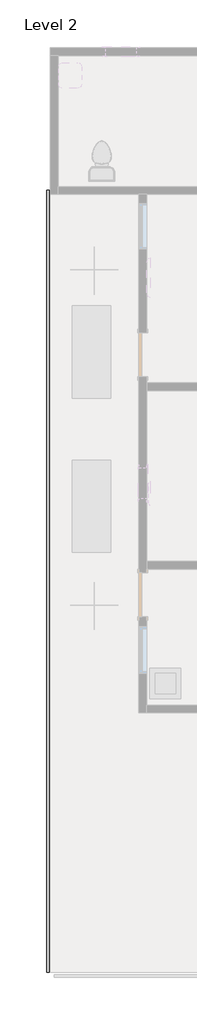
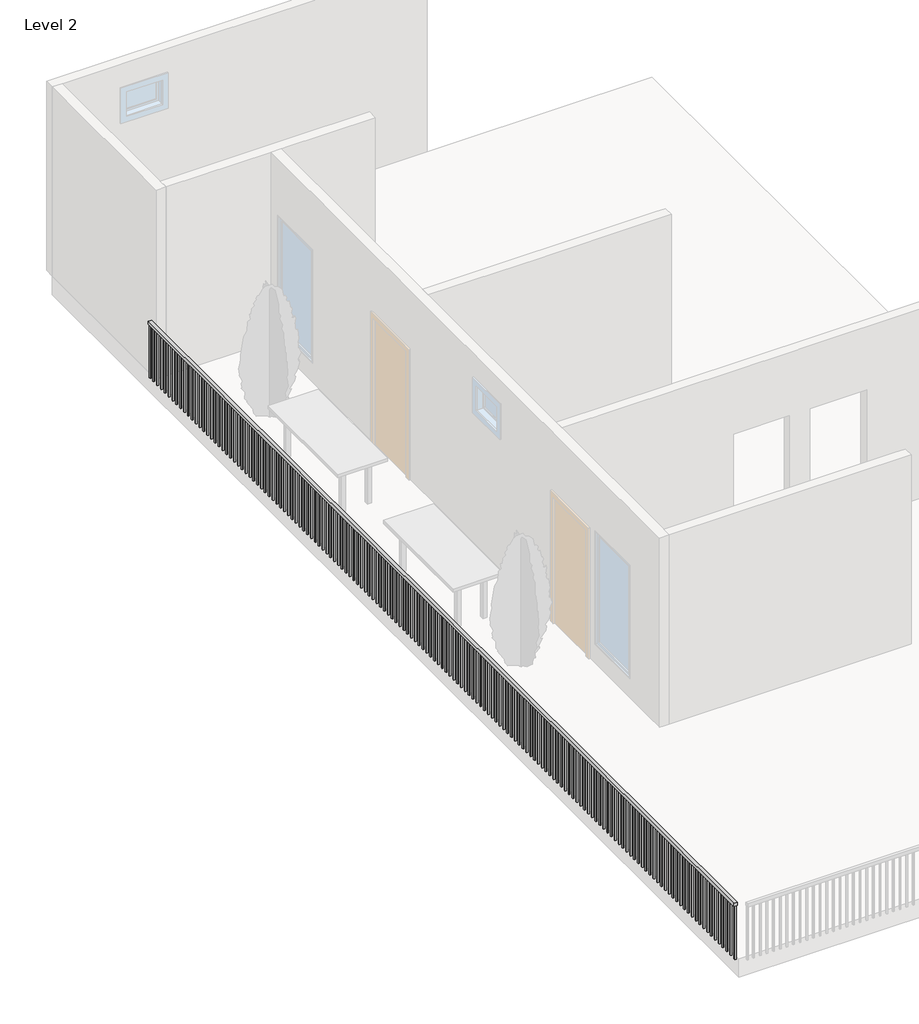
# One storey, part 3 of 4: 1 railing.
"""IFC4 building model written with IfcOpenShell, lengths in millimetres."""

from ifc_helpers import new_model, si_unit, frame, origin, place, context, project, spatial, polyline, outline, extrude, element, save

model = new_model("IFC4")

# Units and contexts
model_context = context("Model", 3, world=origin())
ifc_project = project(units=[si_unit("LENGTHUNIT", "METRE", prefix="MILLI")], contexts=[model_context])

# Site, building, storey
site = spatial("IfcSite", under=ifc_project)
building = spatial("IfcBuilding", under=site)
storey = spatial("IfcBuildingStorey", under=building, Name="Level 2", Elevation=3048.0)

# Railing
placement = place(None, origin())
element("IfcRailing", 1, ObjectType="Handrail - Rectangular", at=placement, inside=storey, context=model_context, shape_type="SweptSolid", body=[
    extrude(outline(polyline([(-12111.260887, 10860.7910469), (-12060.460887, 10860.7910469), (-12060.460887, -4607.8089531), (-12111.260887, -4607.8089531), (-12111.260887, 10860.7910469)])), frame((0.0, 0.0, 3911.6), z_axis=(0.0, 0.0, 1.0), x_axis=(1.0, 0.0, 0.0)), (0.0, 0.0, 1.0), 50.8),
    extrude(outline(polyline([(-12095.385887, -4572.8839531), (-12076.335887, -4572.8839531), (-12076.335887, -4591.9339531), (-12095.385887, -4591.9339531), (-12095.385887, -4572.8839531)])), frame((0.0, 0.0, 3048.0), z_axis=(0.0, 0.0, 1.0), x_axis=(1.0, 0.0, 0.0)), (0.0, 0.0, 1.0), 863.6),
    extrude(outline(polyline([(-12095.385887, -4471.2839531), (-12076.335887, -4471.2839531), (-12076.335887, -4490.3339531), (-12095.385887, -4490.3339531), (-12095.385887, -4471.2839531)])), frame((0.0, 0.0, 3048.0), z_axis=(0.0, 0.0, 1.0), x_axis=(1.0, 0.0, 0.0)), (0.0, 0.0, 1.0), 863.6),
    extrude(outline(polyline([(-12095.385887, -4369.6839531), (-12076.335887, -4369.6839531), (-12076.335887, -4388.7339531), (-12095.385887, -4388.7339531), (-12095.385887, -4369.6839531)])), frame((0.0, 0.0, 3048.0), z_axis=(0.0, 0.0, 1.0), x_axis=(1.0, 0.0, 0.0)), (0.0, 0.0, 1.0), 863.6),
    extrude(outline(polyline([(-12095.385887, -4268.0839531), (-12076.335887, -4268.0839531), (-12076.335887, -4287.1339531), (-12095.385887, -4287.1339531), (-12095.385887, -4268.0839531)])), frame((0.0, 0.0, 3048.0), z_axis=(0.0, 0.0, 1.0), x_axis=(1.0, 0.0, 0.0)), (0.0, 0.0, 1.0), 863.6),
    extrude(outline(polyline([(-12095.385887, -4166.4839531), (-12076.335887, -4166.4839531), (-12076.335887, -4185.5339531), (-12095.385887, -4185.5339531), (-12095.385887, -4166.4839531)])), frame((0.0, 0.0, 3048.0), z_axis=(0.0, 0.0, 1.0), x_axis=(1.0, 0.0, 0.0)), (0.0, 0.0, 1.0), 863.6),
    extrude(outline(polyline([(-12095.385887, -4064.8839531), (-12076.335887, -4064.8839531), (-12076.335887, -4083.9339531), (-12095.385887, -4083.9339531), (-12095.385887, -4064.8839531)])), frame((0.0, 0.0, 3048.0), z_axis=(0.0, 0.0, 1.0), x_axis=(1.0, 0.0, 0.0)), (0.0, 0.0, 1.0), 863.6),
    extrude(outline(polyline([(-12095.385887, -3963.2839531), (-12076.335887, -3963.2839531), (-12076.335887, -3982.3339531), (-12095.385887, -3982.3339531), (-12095.385887, -3963.2839531)])), frame((0.0, 0.0, 3048.0), z_axis=(0.0, 0.0, 1.0), x_axis=(1.0, 0.0, 0.0)), (0.0, 0.0, 1.0), 863.6),
    extrude(outline(polyline([(-12095.385887, -3861.6839531), (-12076.335887, -3861.6839531), (-12076.335887, -3880.7339531), (-12095.385887, -3880.7339531), (-12095.385887, -3861.6839531)])), frame((0.0, 0.0, 3048.0), z_axis=(0.0, 0.0, 1.0), x_axis=(1.0, 0.0, 0.0)), (0.0, 0.0, 1.0), 863.6),
    extrude(outline(polyline([(-12095.385887, -3760.0839531), (-12076.335887, -3760.0839531), (-12076.335887, -3779.1339531), (-12095.385887, -3779.1339531), (-12095.385887, -3760.0839531)])), frame((0.0, 0.0, 3048.0), z_axis=(0.0, 0.0, 1.0), x_axis=(1.0, 0.0, 0.0)), (0.0, 0.0, 1.0), 863.6),
    extrude(outline(polyline([(-12095.385887, -3658.4839531), (-12076.335887, -3658.4839531), (-12076.335887, -3677.5339531), (-12095.385887, -3677.5339531), (-12095.385887, -3658.4839531)])), frame((0.0, 0.0, 3048.0), z_axis=(0.0, 0.0, 1.0), x_axis=(1.0, 0.0, 0.0)), (0.0, 0.0, 1.0), 863.6),
    extrude(outline(polyline([(-12095.385887, -3556.8839531), (-12076.335887, -3556.8839531), (-12076.335887, -3575.9339531), (-12095.385887, -3575.9339531), (-12095.385887, -3556.8839531)])), frame((0.0, 0.0, 3048.0), z_axis=(0.0, 0.0, 1.0), x_axis=(1.0, 0.0, 0.0)), (0.0, 0.0, 1.0), 863.6),
    extrude(outline(polyline([(-12095.385887, -3455.2839531), (-12076.335887, -3455.2839531), (-12076.335887, -3474.3339531), (-12095.385887, -3474.3339531), (-12095.385887, -3455.2839531)])), frame((0.0, 0.0, 3048.0), z_axis=(0.0, 0.0, 1.0), x_axis=(1.0, 0.0, 0.0)), (0.0, 0.0, 1.0), 863.6),
    extrude(outline(polyline([(-12095.385887, -3353.6839531), (-12076.335887, -3353.6839531), (-12076.335887, -3372.7339531), (-12095.385887, -3372.7339531), (-12095.385887, -3353.6839531)])), frame((0.0, 0.0, 3048.0), z_axis=(0.0, 0.0, 1.0), x_axis=(1.0, 0.0, 0.0)), (0.0, 0.0, 1.0), 863.6),
    extrude(outline(polyline([(-12095.385887, -3252.0839531), (-12076.335887, -3252.0839531), (-12076.335887, -3271.1339531), (-12095.385887, -3271.1339531), (-12095.385887, -3252.0839531)])), frame((0.0, 0.0, 3048.0), z_axis=(0.0, 0.0, 1.0), x_axis=(1.0, 0.0, 0.0)), (0.0, 0.0, 1.0), 863.6),
    extrude(outline(polyline([(-12095.385887, -3150.4839531), (-12076.335887, -3150.4839531), (-12076.335887, -3169.5339531), (-12095.385887, -3169.5339531), (-12095.385887, -3150.4839531)])), frame((0.0, 0.0, 3048.0), z_axis=(0.0, 0.0, 1.0), x_axis=(1.0, 0.0, 0.0)), (0.0, 0.0, 1.0), 863.6),
    extrude(outline(polyline([(-12095.385887, -3048.8839531), (-12076.335887, -3048.8839531), (-12076.335887, -3067.9339531), (-12095.385887, -3067.9339531), (-12095.385887, -3048.8839531)])), frame((0.0, 0.0, 3048.0), z_axis=(0.0, 0.0, 1.0), x_axis=(1.0, 0.0, 0.0)), (0.0, 0.0, 1.0), 863.6),
    extrude(outline(polyline([(-12095.385887, -2947.2839531), (-12076.335887, -2947.2839531), (-12076.335887, -2966.3339531), (-12095.385887, -2966.3339531), (-12095.385887, -2947.2839531)])), frame((0.0, 0.0, 3048.0), z_axis=(0.0, 0.0, 1.0), x_axis=(1.0, 0.0, 0.0)), (0.0, 0.0, 1.0), 863.6),
    extrude(outline(polyline([(-12095.385887, -2845.6839531), (-12076.335887, -2845.6839531), (-12076.335887, -2864.7339531), (-12095.385887, -2864.7339531), (-12095.385887, -2845.6839531)])), frame((0.0, 0.0, 3048.0), z_axis=(0.0, 0.0, 1.0), x_axis=(1.0, 0.0, 0.0)), (0.0, 0.0, 1.0), 863.6),
    extrude(outline(polyline([(-12095.385887, -2744.0839531), (-12076.335887, -2744.0839531), (-12076.335887, -2763.1339531), (-12095.385887, -2763.1339531), (-12095.385887, -2744.0839531)])), frame((0.0, 0.0, 3048.0), z_axis=(0.0, 0.0, 1.0), x_axis=(1.0, 0.0, 0.0)), (0.0, 0.0, 1.0), 863.6),
    extrude(outline(polyline([(-12095.385887, -2642.4839531), (-12076.335887, -2642.4839531), (-12076.335887, -2661.5339531), (-12095.385887, -2661.5339531), (-12095.385887, -2642.4839531)])), frame((0.0, 0.0, 3048.0), z_axis=(0.0, 0.0, 1.0), x_axis=(1.0, 0.0, 0.0)), (0.0, 0.0, 1.0), 863.6),
    extrude(outline(polyline([(-12095.385887, -2540.8839531), (-12076.335887, -2540.8839531), (-12076.335887, -2559.9339531), (-12095.385887, -2559.9339531), (-12095.385887, -2540.8839531)])), frame((0.0, 0.0, 3048.0), z_axis=(0.0, 0.0, 1.0), x_axis=(1.0, 0.0, 0.0)), (0.0, 0.0, 1.0), 863.6),
    extrude(outline(polyline([(-12095.385887, -2439.2839531), (-12076.335887, -2439.2839531), (-12076.335887, -2458.3339531), (-12095.385887, -2458.3339531), (-12095.385887, -2439.2839531)])), frame((0.0, 0.0, 3048.0), z_axis=(0.0, 0.0, 1.0), x_axis=(1.0, 0.0, 0.0)), (0.0, 0.0, 1.0), 863.6),
    extrude(outline(polyline([(-12095.385887, -2337.6839531), (-12076.335887, -2337.6839531), (-12076.335887, -2356.7339531), (-12095.385887, -2356.7339531), (-12095.385887, -2337.6839531)])), frame((0.0, 0.0, 3048.0), z_axis=(0.0, 0.0, 1.0), x_axis=(1.0, 0.0, 0.0)), (0.0, 0.0, 1.0), 863.6),
    extrude(outline(polyline([(-12095.385887, -2236.0839531), (-12076.335887, -2236.0839531), (-12076.335887, -2255.1339531), (-12095.385887, -2255.1339531), (-12095.385887, -2236.0839531)])), frame((0.0, 0.0, 3048.0), z_axis=(0.0, 0.0, 1.0), x_axis=(1.0, 0.0, 0.0)), (0.0, 0.0, 1.0), 863.6),
    extrude(outline(polyline([(-12095.385887, -2134.4839531), (-12076.335887, -2134.4839531), (-12076.335887, -2153.5339531), (-12095.385887, -2153.5339531), (-12095.385887, -2134.4839531)])), frame((0.0, 0.0, 3048.0), z_axis=(0.0, 0.0, 1.0), x_axis=(1.0, 0.0, 0.0)), (0.0, 0.0, 1.0), 863.6),
    extrude(outline(polyline([(-12095.385887, -2032.8839531), (-12076.335887, -2032.8839531), (-12076.335887, -2051.9339531), (-12095.385887, -2051.9339531), (-12095.385887, -2032.8839531)])), frame((0.0, 0.0, 3048.0), z_axis=(0.0, 0.0, 1.0), x_axis=(1.0, 0.0, 0.0)), (0.0, 0.0, 1.0), 863.6),
    extrude(outline(polyline([(-12095.385887, -1931.2839531), (-12076.335887, -1931.2839531), (-12076.335887, -1950.3339531), (-12095.385887, -1950.3339531), (-12095.385887, -1931.2839531)])), frame((0.0, 0.0, 3048.0), z_axis=(0.0, 0.0, 1.0), x_axis=(1.0, 0.0, 0.0)), (0.0, 0.0, 1.0), 863.6),
    extrude(outline(polyline([(-12095.385887, -1829.6839531), (-12076.335887, -1829.6839531), (-12076.335887, -1848.7339531), (-12095.385887, -1848.7339531), (-12095.385887, -1829.6839531)])), frame((0.0, 0.0, 3048.0), z_axis=(0.0, 0.0, 1.0), x_axis=(1.0, 0.0, 0.0)), (0.0, 0.0, 1.0), 863.6),
    extrude(outline(polyline([(-12095.385887, -1728.0839531), (-12076.335887, -1728.0839531), (-12076.335887, -1747.1339531), (-12095.385887, -1747.1339531), (-12095.385887, -1728.0839531)])), frame((0.0, 0.0, 3048.0), z_axis=(0.0, 0.0, 1.0), x_axis=(1.0, 0.0, 0.0)), (0.0, 0.0, 1.0), 863.6),
    extrude(outline(polyline([(-12095.385887, -1626.4839531), (-12076.335887, -1626.4839531), (-12076.335887, -1645.5339531), (-12095.385887, -1645.5339531), (-12095.385887, -1626.4839531)])), frame((0.0, 0.0, 3048.0), z_axis=(0.0, 0.0, 1.0), x_axis=(1.0, 0.0, 0.0)), (0.0, 0.0, 1.0), 863.6),
    extrude(outline(polyline([(-12095.385887, -1524.8839531), (-12076.335887, -1524.8839531), (-12076.335887, -1543.9339531), (-12095.385887, -1543.9339531), (-12095.385887, -1524.8839531)])), frame((0.0, 0.0, 3048.0), z_axis=(0.0, 0.0, 1.0), x_axis=(1.0, 0.0, 0.0)), (0.0, 0.0, 1.0), 863.6),
    extrude(outline(polyline([(-12095.385887, -1423.2839531), (-12076.335887, -1423.2839531), (-12076.335887, -1442.3339531), (-12095.385887, -1442.3339531), (-12095.385887, -1423.2839531)])), frame((0.0, 0.0, 3048.0), z_axis=(0.0, 0.0, 1.0), x_axis=(1.0, 0.0, 0.0)), (0.0, 0.0, 1.0), 863.6),
    extrude(outline(polyline([(-12095.385887, -1321.6839531), (-12076.335887, -1321.6839531), (-12076.335887, -1340.7339531), (-12095.385887, -1340.7339531), (-12095.385887, -1321.6839531)])), frame((0.0, 0.0, 3048.0), z_axis=(0.0, 0.0, 1.0), x_axis=(1.0, 0.0, 0.0)), (0.0, 0.0, 1.0), 863.6),
    extrude(outline(polyline([(-12095.385887, -1220.0839531), (-12076.335887, -1220.0839531), (-12076.335887, -1239.1339531), (-12095.385887, -1239.1339531), (-12095.385887, -1220.0839531)])), frame((0.0, 0.0, 3048.0), z_axis=(0.0, 0.0, 1.0), x_axis=(1.0, 0.0, 0.0)), (0.0, 0.0, 1.0), 863.6),
    extrude(outline(polyline([(-12095.385887, -1118.4839531), (-12076.335887, -1118.4839531), (-12076.335887, -1137.5339531), (-12095.385887, -1137.5339531), (-12095.385887, -1118.4839531)])), frame((0.0, 0.0, 3048.0), z_axis=(0.0, 0.0, 1.0), x_axis=(1.0, 0.0, 0.0)), (0.0, 0.0, 1.0), 863.6),
    extrude(outline(polyline([(-12095.385887, -1016.8839531), (-12076.335887, -1016.8839531), (-12076.335887, -1035.9339531), (-12095.385887, -1035.9339531), (-12095.385887, -1016.8839531)])), frame((0.0, 0.0, 3048.0), z_axis=(0.0, 0.0, 1.0), x_axis=(1.0, 0.0, 0.0)), (0.0, 0.0, 1.0), 863.6),
    extrude(outline(polyline([(-12095.385887, -915.2839531), (-12076.335887, -915.2839531), (-12076.335887, -934.3339531), (-12095.385887, -934.3339531), (-12095.385887, -915.2839531)])), frame((0.0, 0.0, 3048.0), z_axis=(0.0, 0.0, 1.0), x_axis=(1.0, 0.0, 0.0)), (0.0, 0.0, 1.0), 863.6),
    extrude(outline(polyline([(-12095.385887, -813.6839531), (-12076.335887, -813.6839531), (-12076.335887, -832.7339531), (-12095.385887, -832.7339531), (-12095.385887, -813.6839531)])), frame((0.0, 0.0, 3048.0), z_axis=(0.0, 0.0, 1.0), x_axis=(1.0, 0.0, 0.0)), (0.0, 0.0, 1.0), 863.6),
    extrude(outline(polyline([(-12095.385887, -712.0839531), (-12076.335887, -712.0839531), (-12076.335887, -731.1339531), (-12095.385887, -731.1339531), (-12095.385887, -712.0839531)])), frame((0.0, 0.0, 3048.0), z_axis=(0.0, 0.0, 1.0), x_axis=(1.0, 0.0, 0.0)), (0.0, 0.0, 1.0), 863.6),
    extrude(outline(polyline([(-12095.385887, -610.4839531), (-12076.335887, -610.4839531), (-12076.335887, -629.5339531), (-12095.385887, -629.5339531), (-12095.385887, -610.4839531)])), frame((0.0, 0.0, 3048.0), z_axis=(0.0, 0.0, 1.0), x_axis=(1.0, 0.0, 0.0)), (0.0, 0.0, 1.0), 863.6),
    extrude(outline(polyline([(-12095.385887, -508.8839531), (-12076.335887, -508.8839531), (-12076.335887, -527.9339531), (-12095.385887, -527.9339531), (-12095.385887, -508.8839531)])), frame((0.0, 0.0, 3048.0), z_axis=(0.0, 0.0, 1.0), x_axis=(1.0, 0.0, 0.0)), (0.0, 0.0, 1.0), 863.6),
    extrude(outline(polyline([(-12095.385887, -407.2839531), (-12076.335887, -407.2839531), (-12076.335887, -426.3339531), (-12095.385887, -426.3339531), (-12095.385887, -407.2839531)])), frame((0.0, 0.0, 3048.0), z_axis=(0.0, 0.0, 1.0), x_axis=(1.0, 0.0, 0.0)), (0.0, 0.0, 1.0), 863.6),
    extrude(outline(polyline([(-12095.385887, -305.6839531), (-12076.335887, -305.6839531), (-12076.335887, -324.7339531), (-12095.385887, -324.7339531), (-12095.385887, -305.6839531)])), frame((0.0, 0.0, 3048.0), z_axis=(0.0, 0.0, 1.0), x_axis=(1.0, 0.0, 0.0)), (0.0, 0.0, 1.0), 863.6),
    extrude(outline(polyline([(-12095.385887, -204.0839531), (-12076.335887, -204.0839531), (-12076.335887, -223.1339531), (-12095.385887, -223.1339531), (-12095.385887, -204.0839531)])), frame((0.0, 0.0, 3048.0), z_axis=(0.0, 0.0, 1.0), x_axis=(1.0, 0.0, 0.0)), (0.0, 0.0, 1.0), 863.6),
    extrude(outline(polyline([(-12095.385887, -102.4839531), (-12076.335887, -102.4839531), (-12076.335887, -121.5339531), (-12095.385887, -121.5339531), (-12095.385887, -102.4839531)])), frame((0.0, 0.0, 3048.0), z_axis=(0.0, 0.0, 1.0), x_axis=(1.0, 0.0, 0.0)), (0.0, 0.0, 1.0), 863.6),
    extrude(outline(polyline([(-12095.385887, -0.8839531), (-12076.335887, -0.8839531), (-12076.335887, -19.9339531), (-12095.385887, -19.9339531), (-12095.385887, -0.8839531)])), frame((0.0, 0.0, 3048.0), z_axis=(0.0, 0.0, 1.0), x_axis=(1.0, 0.0, 0.0)), (0.0, 0.0, 1.0), 863.6),
    extrude(outline(polyline([(-12095.385887, 100.7160469), (-12076.335887, 100.7160469), (-12076.335887, 81.6660469), (-12095.385887, 81.6660469), (-12095.385887, 100.7160469)])), frame((0.0, 0.0, 3048.0), z_axis=(0.0, 0.0, 1.0), x_axis=(1.0, 0.0, 0.0)), (0.0, 0.0, 1.0), 863.6),
    extrude(outline(polyline([(-12095.385887, 202.3160469), (-12076.335887, 202.3160469), (-12076.335887, 183.2660469), (-12095.385887, 183.2660469), (-12095.385887, 202.3160469)])), frame((0.0, 0.0, 3048.0), z_axis=(0.0, 0.0, 1.0), x_axis=(1.0, 0.0, 0.0)), (0.0, 0.0, 1.0), 863.6),
    extrude(outline(polyline([(-12095.385887, 303.9160469), (-12076.335887, 303.9160469), (-12076.335887, 284.8660469), (-12095.385887, 284.8660469), (-12095.385887, 303.9160469)])), frame((0.0, 0.0, 3048.0), z_axis=(0.0, 0.0, 1.0), x_axis=(1.0, 0.0, 0.0)), (0.0, 0.0, 1.0), 863.6),
    extrude(outline(polyline([(-12095.385887, 405.5160469), (-12076.335887, 405.5160469), (-12076.335887, 386.4660469), (-12095.385887, 386.4660469), (-12095.385887, 405.5160469)])), frame((0.0, 0.0, 3048.0), z_axis=(0.0, 0.0, 1.0), x_axis=(1.0, 0.0, 0.0)), (0.0, 0.0, 1.0), 863.6),
    extrude(outline(polyline([(-12095.385887, 507.1160469), (-12076.335887, 507.1160469), (-12076.335887, 488.0660469), (-12095.385887, 488.0660469), (-12095.385887, 507.1160469)])), frame((0.0, 0.0, 3048.0), z_axis=(0.0, 0.0, 1.0), x_axis=(1.0, 0.0, 0.0)), (0.0, 0.0, 1.0), 863.6),
    extrude(outline(polyline([(-12095.385887, 608.7160469), (-12076.335887, 608.7160469), (-12076.335887, 589.6660469), (-12095.385887, 589.6660469), (-12095.385887, 608.7160469)])), frame((0.0, 0.0, 3048.0), z_axis=(0.0, 0.0, 1.0), x_axis=(1.0, 0.0, 0.0)), (0.0, 0.0, 1.0), 863.6),
    extrude(outline(polyline([(-12095.385887, 710.3160469), (-12076.335887, 710.3160469), (-12076.335887, 691.2660469), (-12095.385887, 691.2660469), (-12095.385887, 710.3160469)])), frame((0.0, 0.0, 3048.0), z_axis=(0.0, 0.0, 1.0), x_axis=(1.0, 0.0, 0.0)), (0.0, 0.0, 1.0), 863.6),
    extrude(outline(polyline([(-12095.385887, 811.9160469), (-12076.335887, 811.9160469), (-12076.335887, 792.8660469), (-12095.385887, 792.8660469), (-12095.385887, 811.9160469)])), frame((0.0, 0.0, 3048.0), z_axis=(0.0, 0.0, 1.0), x_axis=(1.0, 0.0, 0.0)), (0.0, 0.0, 1.0), 863.6),
    extrude(outline(polyline([(-12095.385887, 913.5160469), (-12076.335887, 913.5160469), (-12076.335887, 894.4660469), (-12095.385887, 894.4660469), (-12095.385887, 913.5160469)])), frame((0.0, 0.0, 3048.0), z_axis=(0.0, 0.0, 1.0), x_axis=(1.0, 0.0, 0.0)), (0.0, 0.0, 1.0), 863.6),
    extrude(outline(polyline([(-12095.385887, 1015.1160469), (-12076.335887, 1015.1160469), (-12076.335887, 996.0660469), (-12095.385887, 996.0660469), (-12095.385887, 1015.1160469)])), frame((0.0, 0.0, 3048.0), z_axis=(0.0, 0.0, 1.0), x_axis=(1.0, 0.0, 0.0)), (0.0, 0.0, 1.0), 863.6),
    extrude(outline(polyline([(-12095.385887, 1116.7160469), (-12076.335887, 1116.7160469), (-12076.335887, 1097.6660469), (-12095.385887, 1097.6660469), (-12095.385887, 1116.7160469)])), frame((0.0, 0.0, 3048.0), z_axis=(0.0, 0.0, 1.0), x_axis=(1.0, 0.0, 0.0)), (0.0, 0.0, 1.0), 863.6),
    extrude(outline(polyline([(-12095.385887, 1218.3160469), (-12076.335887, 1218.3160469), (-12076.335887, 1199.2660469), (-12095.385887, 1199.2660469), (-12095.385887, 1218.3160469)])), frame((0.0, 0.0, 3048.0), z_axis=(0.0, 0.0, 1.0), x_axis=(1.0, 0.0, 0.0)), (0.0, 0.0, 1.0), 863.6),
    extrude(outline(polyline([(-12095.385887, 1319.9160469), (-12076.335887, 1319.9160469), (-12076.335887, 1300.8660469), (-12095.385887, 1300.8660469), (-12095.385887, 1319.9160469)])), frame((0.0, 0.0, 3048.0), z_axis=(0.0, 0.0, 1.0), x_axis=(1.0, 0.0, 0.0)), (0.0, 0.0, 1.0), 863.6),
    extrude(outline(polyline([(-12095.385887, 1421.5160469), (-12076.335887, 1421.5160469), (-12076.335887, 1402.4660469), (-12095.385887, 1402.4660469), (-12095.385887, 1421.5160469)])), frame((0.0, 0.0, 3048.0), z_axis=(0.0, 0.0, 1.0), x_axis=(1.0, 0.0, 0.0)), (0.0, 0.0, 1.0), 863.6),
    extrude(outline(polyline([(-12095.385887, 1523.1160469), (-12076.335887, 1523.1160469), (-12076.335887, 1504.0660469), (-12095.385887, 1504.0660469), (-12095.385887, 1523.1160469)])), frame((0.0, 0.0, 3048.0), z_axis=(0.0, 0.0, 1.0), x_axis=(1.0, 0.0, 0.0)), (0.0, 0.0, 1.0), 863.6),
    extrude(outline(polyline([(-12095.385887, 1624.7160469), (-12076.335887, 1624.7160469), (-12076.335887, 1605.6660469), (-12095.385887, 1605.6660469), (-12095.385887, 1624.7160469)])), frame((0.0, 0.0, 3048.0), z_axis=(0.0, 0.0, 1.0), x_axis=(1.0, 0.0, 0.0)), (0.0, 0.0, 1.0), 863.6),
    extrude(outline(polyline([(-12095.385887, 1726.3160469), (-12076.335887, 1726.3160469), (-12076.335887, 1707.2660469), (-12095.385887, 1707.2660469), (-12095.385887, 1726.3160469)])), frame((0.0, 0.0, 3048.0), z_axis=(0.0, 0.0, 1.0), x_axis=(1.0, 0.0, 0.0)), (0.0, 0.0, 1.0), 863.6),
    extrude(outline(polyline([(-12095.385887, 1827.9160469), (-12076.335887, 1827.9160469), (-12076.335887, 1808.8660469), (-12095.385887, 1808.8660469), (-12095.385887, 1827.9160469)])), frame((0.0, 0.0, 3048.0), z_axis=(0.0, 0.0, 1.0), x_axis=(1.0, 0.0, 0.0)), (0.0, 0.0, 1.0), 863.6),
    extrude(outline(polyline([(-12095.385887, 1929.5160469), (-12076.335887, 1929.5160469), (-12076.335887, 1910.4660469), (-12095.385887, 1910.4660469), (-12095.385887, 1929.5160469)])), frame((0.0, 0.0, 3048.0), z_axis=(0.0, 0.0, 1.0), x_axis=(1.0, 0.0, 0.0)), (0.0, 0.0, 1.0), 863.6),
    extrude(outline(polyline([(-12095.385887, 2031.1160469), (-12076.335887, 2031.1160469), (-12076.335887, 2012.0660469), (-12095.385887, 2012.0660469), (-12095.385887, 2031.1160469)])), frame((0.0, 0.0, 3048.0), z_axis=(0.0, 0.0, 1.0), x_axis=(1.0, 0.0, 0.0)), (0.0, 0.0, 1.0), 863.6),
    extrude(outline(polyline([(-12095.385887, 2132.7160469), (-12076.335887, 2132.7160469), (-12076.335887, 2113.6660469), (-12095.385887, 2113.6660469), (-12095.385887, 2132.7160469)])), frame((0.0, 0.0, 3048.0), z_axis=(0.0, 0.0, 1.0), x_axis=(1.0, 0.0, 0.0)), (0.0, 0.0, 1.0), 863.6),
    extrude(outline(polyline([(-12095.385887, 2234.3160469), (-12076.335887, 2234.3160469), (-12076.335887, 2215.2660469), (-12095.385887, 2215.2660469), (-12095.385887, 2234.3160469)])), frame((0.0, 0.0, 3048.0), z_axis=(0.0, 0.0, 1.0), x_axis=(1.0, 0.0, 0.0)), (0.0, 0.0, 1.0), 863.6),
    extrude(outline(polyline([(-12095.385887, 2335.9160469), (-12076.335887, 2335.9160469), (-12076.335887, 2316.8660469), (-12095.385887, 2316.8660469), (-12095.385887, 2335.9160469)])), frame((0.0, 0.0, 3048.0), z_axis=(0.0, 0.0, 1.0), x_axis=(1.0, 0.0, 0.0)), (0.0, 0.0, 1.0), 863.6),
    extrude(outline(polyline([(-12095.385887, 2437.5160469), (-12076.335887, 2437.5160469), (-12076.335887, 2418.4660469), (-12095.385887, 2418.4660469), (-12095.385887, 2437.5160469)])), frame((0.0, 0.0, 3048.0), z_axis=(0.0, 0.0, 1.0), x_axis=(1.0, 0.0, 0.0)), (0.0, 0.0, 1.0), 863.6),
    extrude(outline(polyline([(-12095.385887, 2539.1160469), (-12076.335887, 2539.1160469), (-12076.335887, 2520.0660469), (-12095.385887, 2520.0660469), (-12095.385887, 2539.1160469)])), frame((0.0, 0.0, 3048.0), z_axis=(0.0, 0.0, 1.0), x_axis=(1.0, 0.0, 0.0)), (0.0, 0.0, 1.0), 863.6),
    extrude(outline(polyline([(-12095.385887, 2640.7160469), (-12076.335887, 2640.7160469), (-12076.335887, 2621.6660469), (-12095.385887, 2621.6660469), (-12095.385887, 2640.7160469)])), frame((0.0, 0.0, 3048.0), z_axis=(0.0, 0.0, 1.0), x_axis=(1.0, 0.0, 0.0)), (0.0, 0.0, 1.0), 863.6),
    extrude(outline(polyline([(-12095.385887, 2742.3160469), (-12076.335887, 2742.3160469), (-12076.335887, 2723.2660469), (-12095.385887, 2723.2660469), (-12095.385887, 2742.3160469)])), frame((0.0, 0.0, 3048.0), z_axis=(0.0, 0.0, 1.0), x_axis=(1.0, 0.0, 0.0)), (0.0, 0.0, 1.0), 863.6),
    extrude(outline(polyline([(-12095.385887, 2843.9160469), (-12076.335887, 2843.9160469), (-12076.335887, 2824.8660469), (-12095.385887, 2824.8660469), (-12095.385887, 2843.9160469)])), frame((0.0, 0.0, 3048.0), z_axis=(0.0, 0.0, 1.0), x_axis=(1.0, 0.0, 0.0)), (0.0, 0.0, 1.0), 863.6),
    extrude(outline(polyline([(-12095.385887, 2945.5160469), (-12076.335887, 2945.5160469), (-12076.335887, 2926.4660469), (-12095.385887, 2926.4660469), (-12095.385887, 2945.5160469)])), frame((0.0, 0.0, 3048.0), z_axis=(0.0, 0.0, 1.0), x_axis=(1.0, 0.0, 0.0)), (0.0, 0.0, 1.0), 863.6),
    extrude(outline(polyline([(-12095.385887, 3047.1160469), (-12076.335887, 3047.1160469), (-12076.335887, 3028.0660469), (-12095.385887, 3028.0660469), (-12095.385887, 3047.1160469)])), frame((0.0, 0.0, 3048.0), z_axis=(0.0, 0.0, 1.0), x_axis=(1.0, 0.0, 0.0)), (0.0, 0.0, 1.0), 863.6),
    extrude(outline(polyline([(-12095.385887, 3148.7160469), (-12076.335887, 3148.7160469), (-12076.335887, 3129.6660469), (-12095.385887, 3129.6660469), (-12095.385887, 3148.7160469)])), frame((0.0, 0.0, 3048.0), z_axis=(0.0, 0.0, 1.0), x_axis=(1.0, 0.0, 0.0)), (0.0, 0.0, 1.0), 863.6),
    extrude(outline(polyline([(-12095.385887, 3250.3160469), (-12076.335887, 3250.3160469), (-12076.335887, 3231.2660469), (-12095.385887, 3231.2660469), (-12095.385887, 3250.3160469)])), frame((0.0, 0.0, 3048.0), z_axis=(0.0, 0.0, 1.0), x_axis=(1.0, 0.0, 0.0)), (0.0, 0.0, 1.0), 863.6),
    extrude(outline(polyline([(-12095.385887, 3351.9160469), (-12076.335887, 3351.9160469), (-12076.335887, 3332.8660469), (-12095.385887, 3332.8660469), (-12095.385887, 3351.9160469)])), frame((0.0, 0.0, 3048.0), z_axis=(0.0, 0.0, 1.0), x_axis=(1.0, 0.0, 0.0)), (0.0, 0.0, 1.0), 863.6),
    extrude(outline(polyline([(-12095.385887, 3453.5160469), (-12076.335887, 3453.5160469), (-12076.335887, 3434.4660469), (-12095.385887, 3434.4660469), (-12095.385887, 3453.5160469)])), frame((0.0, 0.0, 3048.0), z_axis=(0.0, 0.0, 1.0), x_axis=(1.0, 0.0, 0.0)), (0.0, 0.0, 1.0), 863.6),
    extrude(outline(polyline([(-12095.385887, 3555.1160469), (-12076.335887, 3555.1160469), (-12076.335887, 3536.0660469), (-12095.385887, 3536.0660469), (-12095.385887, 3555.1160469)])), frame((0.0, 0.0, 3048.0), z_axis=(0.0, 0.0, 1.0), x_axis=(1.0, 0.0, 0.0)), (0.0, 0.0, 1.0), 863.6),
    extrude(outline(polyline([(-12095.385887, 3656.7160469), (-12076.335887, 3656.7160469), (-12076.335887, 3637.6660469), (-12095.385887, 3637.6660469), (-12095.385887, 3656.7160469)])), frame((0.0, 0.0, 3048.0), z_axis=(0.0, 0.0, 1.0), x_axis=(1.0, 0.0, 0.0)), (0.0, 0.0, 1.0), 863.6),
    extrude(outline(polyline([(-12095.385887, 3758.3160469), (-12076.335887, 3758.3160469), (-12076.335887, 3739.2660469), (-12095.385887, 3739.2660469), (-12095.385887, 3758.3160469)])), frame((0.0, 0.0, 3048.0), z_axis=(0.0, 0.0, 1.0), x_axis=(1.0, 0.0, 0.0)), (0.0, 0.0, 1.0), 863.6),
    extrude(outline(polyline([(-12095.385887, 3859.9160469), (-12076.335887, 3859.9160469), (-12076.335887, 3840.8660469), (-12095.385887, 3840.8660469), (-12095.385887, 3859.9160469)])), frame((0.0, 0.0, 3048.0), z_axis=(0.0, 0.0, 1.0), x_axis=(1.0, 0.0, 0.0)), (0.0, 0.0, 1.0), 863.6),
    extrude(outline(polyline([(-12095.385887, 3961.5160469), (-12076.335887, 3961.5160469), (-12076.335887, 3942.4660469), (-12095.385887, 3942.4660469), (-12095.385887, 3961.5160469)])), frame((0.0, 0.0, 3048.0), z_axis=(0.0, 0.0, 1.0), x_axis=(1.0, 0.0, 0.0)), (0.0, 0.0, 1.0), 863.6),
    extrude(outline(polyline([(-12095.385887, 4063.1160469), (-12076.335887, 4063.1160469), (-12076.335887, 4044.0660469), (-12095.385887, 4044.0660469), (-12095.385887, 4063.1160469)])), frame((0.0, 0.0, 3048.0), z_axis=(0.0, 0.0, 1.0), x_axis=(1.0, 0.0, 0.0)), (0.0, 0.0, 1.0), 863.6),
    extrude(outline(polyline([(-12095.385887, 4164.7160469), (-12076.335887, 4164.7160469), (-12076.335887, 4145.6660469), (-12095.385887, 4145.6660469), (-12095.385887, 4164.7160469)])), frame((0.0, 0.0, 3048.0), z_axis=(0.0, 0.0, 1.0), x_axis=(1.0, 0.0, 0.0)), (0.0, 0.0, 1.0), 863.6),
    extrude(outline(polyline([(-12095.385887, 4266.3160469), (-12076.335887, 4266.3160469), (-12076.335887, 4247.2660469), (-12095.385887, 4247.2660469), (-12095.385887, 4266.3160469)])), frame((0.0, 0.0, 3048.0), z_axis=(0.0, 0.0, 1.0), x_axis=(1.0, 0.0, 0.0)), (0.0, 0.0, 1.0), 863.6),
    extrude(outline(polyline([(-12095.385887, 4367.9160469), (-12076.335887, 4367.9160469), (-12076.335887, 4348.8660469), (-12095.385887, 4348.8660469), (-12095.385887, 4367.9160469)])), frame((0.0, 0.0, 3048.0), z_axis=(0.0, 0.0, 1.0), x_axis=(1.0, 0.0, 0.0)), (0.0, 0.0, 1.0), 863.6),
    extrude(outline(polyline([(-12095.385887, 4469.5160469), (-12076.335887, 4469.5160469), (-12076.335887, 4450.4660469), (-12095.385887, 4450.4660469), (-12095.385887, 4469.5160469)])), frame((0.0, 0.0, 3048.0), z_axis=(0.0, 0.0, 1.0), x_axis=(1.0, 0.0, 0.0)), (0.0, 0.0, 1.0), 863.6),
    extrude(outline(polyline([(-12095.385887, 4571.1160469), (-12076.335887, 4571.1160469), (-12076.335887, 4552.0660469), (-12095.385887, 4552.0660469), (-12095.385887, 4571.1160469)])), frame((0.0, 0.0, 3048.0), z_axis=(0.0, 0.0, 1.0), x_axis=(1.0, 0.0, 0.0)), (0.0, 0.0, 1.0), 863.6),
    extrude(outline(polyline([(-12095.385887, 4672.7160469), (-12076.335887, 4672.7160469), (-12076.335887, 4653.6660469), (-12095.385887, 4653.6660469), (-12095.385887, 4672.7160469)])), frame((0.0, 0.0, 3048.0), z_axis=(0.0, 0.0, 1.0), x_axis=(1.0, 0.0, 0.0)), (0.0, 0.0, 1.0), 863.6),
    extrude(outline(polyline([(-12095.385887, 4774.3160469), (-12076.335887, 4774.3160469), (-12076.335887, 4755.2660469), (-12095.385887, 4755.2660469), (-12095.385887, 4774.3160469)])), frame((0.0, 0.0, 3048.0), z_axis=(0.0, 0.0, 1.0), x_axis=(1.0, 0.0, 0.0)), (0.0, 0.0, 1.0), 863.6),
    extrude(outline(polyline([(-12095.385887, 4875.9160469), (-12076.335887, 4875.9160469), (-12076.335887, 4856.8660469), (-12095.385887, 4856.8660469), (-12095.385887, 4875.9160469)])), frame((0.0, 0.0, 3048.0), z_axis=(0.0, 0.0, 1.0), x_axis=(1.0, 0.0, 0.0)), (0.0, 0.0, 1.0), 863.6),
    extrude(outline(polyline([(-12095.385887, 4977.5160469), (-12076.335887, 4977.5160469), (-12076.335887, 4958.4660469), (-12095.385887, 4958.4660469), (-12095.385887, 4977.5160469)])), frame((0.0, 0.0, 3048.0), z_axis=(0.0, 0.0, 1.0), x_axis=(1.0, 0.0, 0.0)), (0.0, 0.0, 1.0), 863.6),
    extrude(outline(polyline([(-12095.385887, 5079.1160469), (-12076.335887, 5079.1160469), (-12076.335887, 5060.0660469), (-12095.385887, 5060.0660469), (-12095.385887, 5079.1160469)])), frame((0.0, 0.0, 3048.0), z_axis=(0.0, 0.0, 1.0), x_axis=(1.0, 0.0, 0.0)), (0.0, 0.0, 1.0), 863.6),
    extrude(outline(polyline([(-12095.385887, 5180.7160469), (-12076.335887, 5180.7160469), (-12076.335887, 5161.6660469), (-12095.385887, 5161.6660469), (-12095.385887, 5180.7160469)])), frame((0.0, 0.0, 3048.0), z_axis=(0.0, 0.0, 1.0), x_axis=(1.0, 0.0, 0.0)), (0.0, 0.0, 1.0), 863.6),
    extrude(outline(polyline([(-12095.385887, 5282.3160469), (-12076.335887, 5282.3160469), (-12076.335887, 5263.2660469), (-12095.385887, 5263.2660469), (-12095.385887, 5282.3160469)])), frame((0.0, 0.0, 3048.0), z_axis=(0.0, 0.0, 1.0), x_axis=(1.0, 0.0, 0.0)), (0.0, 0.0, 1.0), 863.6),
    extrude(outline(polyline([(-12095.385887, 5383.9160469), (-12076.335887, 5383.9160469), (-12076.335887, 5364.8660469), (-12095.385887, 5364.8660469), (-12095.385887, 5383.9160469)])), frame((0.0, 0.0, 3048.0), z_axis=(0.0, 0.0, 1.0), x_axis=(1.0, 0.0, 0.0)), (0.0, 0.0, 1.0), 863.6),
    extrude(outline(polyline([(-12095.385887, 5485.5160469), (-12076.335887, 5485.5160469), (-12076.335887, 5466.4660469), (-12095.385887, 5466.4660469), (-12095.385887, 5485.5160469)])), frame((0.0, 0.0, 3048.0), z_axis=(0.0, 0.0, 1.0), x_axis=(1.0, 0.0, 0.0)), (0.0, 0.0, 1.0), 863.6),
    extrude(outline(polyline([(-12095.385887, 5587.1160469), (-12076.335887, 5587.1160469), (-12076.335887, 5568.0660469), (-12095.385887, 5568.0660469), (-12095.385887, 5587.1160469)])), frame((0.0, 0.0, 3048.0), z_axis=(0.0, 0.0, 1.0), x_axis=(1.0, 0.0, 0.0)), (0.0, 0.0, 1.0), 863.6),
    extrude(outline(polyline([(-12095.385887, 5688.7160469), (-12076.335887, 5688.7160469), (-12076.335887, 5669.6660469), (-12095.385887, 5669.6660469), (-12095.385887, 5688.7160469)])), frame((0.0, 0.0, 3048.0), z_axis=(0.0, 0.0, 1.0), x_axis=(1.0, 0.0, 0.0)), (0.0, 0.0, 1.0), 863.6),
    extrude(outline(polyline([(-12095.385887, 5790.3160469), (-12076.335887, 5790.3160469), (-12076.335887, 5771.2660469), (-12095.385887, 5771.2660469), (-12095.385887, 5790.3160469)])), frame((0.0, 0.0, 3048.0), z_axis=(0.0, 0.0, 1.0), x_axis=(1.0, 0.0, 0.0)), (0.0, 0.0, 1.0), 863.6),
    extrude(outline(polyline([(-12095.385887, 5891.9160469), (-12076.335887, 5891.9160469), (-12076.335887, 5872.8660469), (-12095.385887, 5872.8660469), (-12095.385887, 5891.9160469)])), frame((0.0, 0.0, 3048.0), z_axis=(0.0, 0.0, 1.0), x_axis=(1.0, 0.0, 0.0)), (0.0, 0.0, 1.0), 863.6),
    extrude(outline(polyline([(-12095.385887, 5993.5160469), (-12076.335887, 5993.5160469), (-12076.335887, 5974.4660469), (-12095.385887, 5974.4660469), (-12095.385887, 5993.5160469)])), frame((0.0, 0.0, 3048.0), z_axis=(0.0, 0.0, 1.0), x_axis=(1.0, 0.0, 0.0)), (0.0, 0.0, 1.0), 863.6),
    extrude(outline(polyline([(-12095.385887, 6095.1160469), (-12076.335887, 6095.1160469), (-12076.335887, 6076.0660469), (-12095.385887, 6076.0660469), (-12095.385887, 6095.1160469)])), frame((0.0, 0.0, 3048.0), z_axis=(0.0, 0.0, 1.0), x_axis=(1.0, 0.0, 0.0)), (0.0, 0.0, 1.0), 863.6),
    extrude(outline(polyline([(-12095.385887, 6196.7160469), (-12076.335887, 6196.7160469), (-12076.335887, 6177.6660469), (-12095.385887, 6177.6660469), (-12095.385887, 6196.7160469)])), frame((0.0, 0.0, 3048.0), z_axis=(0.0, 0.0, 1.0), x_axis=(1.0, 0.0, 0.0)), (0.0, 0.0, 1.0), 863.6),
    extrude(outline(polyline([(-12095.385887, 6298.3160469), (-12076.335887, 6298.3160469), (-12076.335887, 6279.2660469), (-12095.385887, 6279.2660469), (-12095.385887, 6298.3160469)])), frame((0.0, 0.0, 3048.0), z_axis=(0.0, 0.0, 1.0), x_axis=(1.0, 0.0, 0.0)), (0.0, 0.0, 1.0), 863.6),
    extrude(outline(polyline([(-12095.385887, 6399.9160469), (-12076.335887, 6399.9160469), (-12076.335887, 6380.8660469), (-12095.385887, 6380.8660469), (-12095.385887, 6399.9160469)])), frame((0.0, 0.0, 3048.0), z_axis=(0.0, 0.0, 1.0), x_axis=(1.0, 0.0, 0.0)), (0.0, 0.0, 1.0), 863.6),
    extrude(outline(polyline([(-12095.385887, 6501.5160469), (-12076.335887, 6501.5160469), (-12076.335887, 6482.4660469), (-12095.385887, 6482.4660469), (-12095.385887, 6501.5160469)])), frame((0.0, 0.0, 3048.0), z_axis=(0.0, 0.0, 1.0), x_axis=(1.0, 0.0, 0.0)), (0.0, 0.0, 1.0), 863.6),
    extrude(outline(polyline([(-12095.385887, 6603.1160469), (-12076.335887, 6603.1160469), (-12076.335887, 6584.0660469), (-12095.385887, 6584.0660469), (-12095.385887, 6603.1160469)])), frame((0.0, 0.0, 3048.0), z_axis=(0.0, 0.0, 1.0), x_axis=(1.0, 0.0, 0.0)), (0.0, 0.0, 1.0), 863.6),
    extrude(outline(polyline([(-12095.385887, 6704.7160469), (-12076.335887, 6704.7160469), (-12076.335887, 6685.6660469), (-12095.385887, 6685.6660469), (-12095.385887, 6704.7160469)])), frame((0.0, 0.0, 3048.0), z_axis=(0.0, 0.0, 1.0), x_axis=(1.0, 0.0, 0.0)), (0.0, 0.0, 1.0), 863.6),
    extrude(outline(polyline([(-12095.385887, 6806.3160469), (-12076.335887, 6806.3160469), (-12076.335887, 6787.2660469), (-12095.385887, 6787.2660469), (-12095.385887, 6806.3160469)])), frame((0.0, 0.0, 3048.0), z_axis=(0.0, 0.0, 1.0), x_axis=(1.0, 0.0, 0.0)), (0.0, 0.0, 1.0), 863.6),
    extrude(outline(polyline([(-12095.385887, 6907.9160469), (-12076.335887, 6907.9160469), (-12076.335887, 6888.8660469), (-12095.385887, 6888.8660469), (-12095.385887, 6907.9160469)])), frame((0.0, 0.0, 3048.0), z_axis=(0.0, 0.0, 1.0), x_axis=(1.0, 0.0, 0.0)), (0.0, 0.0, 1.0), 863.6),
    extrude(outline(polyline([(-12095.385887, 7009.5160469), (-12076.335887, 7009.5160469), (-12076.335887, 6990.4660469), (-12095.385887, 6990.4660469), (-12095.385887, 7009.5160469)])), frame((0.0, 0.0, 3048.0), z_axis=(0.0, 0.0, 1.0), x_axis=(1.0, 0.0, 0.0)), (0.0, 0.0, 1.0), 863.6),
    extrude(outline(polyline([(-12095.385887, 7111.1160469), (-12076.335887, 7111.1160469), (-12076.335887, 7092.0660469), (-12095.385887, 7092.0660469), (-12095.385887, 7111.1160469)])), frame((0.0, 0.0, 3048.0), z_axis=(0.0, 0.0, 1.0), x_axis=(1.0, 0.0, 0.0)), (0.0, 0.0, 1.0), 863.6),
    extrude(outline(polyline([(-12095.385887, 7212.7160469), (-12076.335887, 7212.7160469), (-12076.335887, 7193.6660469), (-12095.385887, 7193.6660469), (-12095.385887, 7212.7160469)])), frame((0.0, 0.0, 3048.0), z_axis=(0.0, 0.0, 1.0), x_axis=(1.0, 0.0, 0.0)), (0.0, 0.0, 1.0), 863.6),
    extrude(outline(polyline([(-12095.385887, 7314.3160469), (-12076.335887, 7314.3160469), (-12076.335887, 7295.2660469), (-12095.385887, 7295.2660469), (-12095.385887, 7314.3160469)])), frame((0.0, 0.0, 3048.0), z_axis=(0.0, 0.0, 1.0), x_axis=(1.0, 0.0, 0.0)), (0.0, 0.0, 1.0), 863.6),
    extrude(outline(polyline([(-12095.385887, 7415.9160469), (-12076.335887, 7415.9160469), (-12076.335887, 7396.8660469), (-12095.385887, 7396.8660469), (-12095.385887, 7415.9160469)])), frame((0.0, 0.0, 3048.0), z_axis=(0.0, 0.0, 1.0), x_axis=(1.0, 0.0, 0.0)), (0.0, 0.0, 1.0), 863.6),
    extrude(outline(polyline([(-12095.385887, 7517.5160469), (-12076.335887, 7517.5160469), (-12076.335887, 7498.4660469), (-12095.385887, 7498.4660469), (-12095.385887, 7517.5160469)])), frame((0.0, 0.0, 3048.0), z_axis=(0.0, 0.0, 1.0), x_axis=(1.0, 0.0, 0.0)), (0.0, 0.0, 1.0), 863.6),
    extrude(outline(polyline([(-12095.385887, 7619.1160469), (-12076.335887, 7619.1160469), (-12076.335887, 7600.0660469), (-12095.385887, 7600.0660469), (-12095.385887, 7619.1160469)])), frame((0.0, 0.0, 3048.0), z_axis=(0.0, 0.0, 1.0), x_axis=(1.0, 0.0, 0.0)), (0.0, 0.0, 1.0), 863.6),
    extrude(outline(polyline([(-12095.385887, 7720.7160469), (-12076.335887, 7720.7160469), (-12076.335887, 7701.6660469), (-12095.385887, 7701.6660469), (-12095.385887, 7720.7160469)])), frame((0.0, 0.0, 3048.0), z_axis=(0.0, 0.0, 1.0), x_axis=(1.0, 0.0, 0.0)), (0.0, 0.0, 1.0), 863.6),
    extrude(outline(polyline([(-12095.385887, 7822.3160469), (-12076.335887, 7822.3160469), (-12076.335887, 7803.2660469), (-12095.385887, 7803.2660469), (-12095.385887, 7822.3160469)])), frame((0.0, 0.0, 3048.0), z_axis=(0.0, 0.0, 1.0), x_axis=(1.0, 0.0, 0.0)), (0.0, 0.0, 1.0), 863.6),
    extrude(outline(polyline([(-12095.385887, 7923.9160469), (-12076.335887, 7923.9160469), (-12076.335887, 7904.8660469), (-12095.385887, 7904.8660469), (-12095.385887, 7923.9160469)])), frame((0.0, 0.0, 3048.0), z_axis=(0.0, 0.0, 1.0), x_axis=(1.0, 0.0, 0.0)), (0.0, 0.0, 1.0), 863.6),
    extrude(outline(polyline([(-12095.385887, 8025.5160469), (-12076.335887, 8025.5160469), (-12076.335887, 8006.4660469), (-12095.385887, 8006.4660469), (-12095.385887, 8025.5160469)])), frame((0.0, 0.0, 3048.0), z_axis=(0.0, 0.0, 1.0), x_axis=(1.0, 0.0, 0.0)), (0.0, 0.0, 1.0), 863.6),
    extrude(outline(polyline([(-12095.385887, 8127.1160469), (-12076.335887, 8127.1160469), (-12076.335887, 8108.0660469), (-12095.385887, 8108.0660469), (-12095.385887, 8127.1160469)])), frame((0.0, 0.0, 3048.0), z_axis=(0.0, 0.0, 1.0), x_axis=(1.0, 0.0, 0.0)), (0.0, 0.0, 1.0), 863.6),
    extrude(outline(polyline([(-12095.385887, 8228.7160469), (-12076.335887, 8228.7160469), (-12076.335887, 8209.6660469), (-12095.385887, 8209.6660469), (-12095.385887, 8228.7160469)])), frame((0.0, 0.0, 3048.0), z_axis=(0.0, 0.0, 1.0), x_axis=(1.0, 0.0, 0.0)), (0.0, 0.0, 1.0), 863.6),
    extrude(outline(polyline([(-12095.385887, 8330.3160469), (-12076.335887, 8330.3160469), (-12076.335887, 8311.2660469), (-12095.385887, 8311.2660469), (-12095.385887, 8330.3160469)])), frame((0.0, 0.0, 3048.0), z_axis=(0.0, 0.0, 1.0), x_axis=(1.0, 0.0, 0.0)), (0.0, 0.0, 1.0), 863.6),
    extrude(outline(polyline([(-12095.385887, 8431.9160469), (-12076.335887, 8431.9160469), (-12076.335887, 8412.8660469), (-12095.385887, 8412.8660469), (-12095.385887, 8431.9160469)])), frame((0.0, 0.0, 3048.0), z_axis=(0.0, 0.0, 1.0), x_axis=(1.0, 0.0, 0.0)), (0.0, 0.0, 1.0), 863.6),
    extrude(outline(polyline([(-12095.385887, 8533.5160469), (-12076.335887, 8533.5160469), (-12076.335887, 8514.4660469), (-12095.385887, 8514.4660469), (-12095.385887, 8533.5160469)])), frame((0.0, 0.0, 3048.0), z_axis=(0.0, 0.0, 1.0), x_axis=(1.0, 0.0, 0.0)), (0.0, 0.0, 1.0), 863.6),
    extrude(outline(polyline([(-12095.385887, 8635.1160469), (-12076.335887, 8635.1160469), (-12076.335887, 8616.0660469), (-12095.385887, 8616.0660469), (-12095.385887, 8635.1160469)])), frame((0.0, 0.0, 3048.0), z_axis=(0.0, 0.0, 1.0), x_axis=(1.0, 0.0, 0.0)), (0.0, 0.0, 1.0), 863.6),
    extrude(outline(polyline([(-12095.385887, 8736.7160469), (-12076.335887, 8736.7160469), (-12076.335887, 8717.6660469), (-12095.385887, 8717.6660469), (-12095.385887, 8736.7160469)])), frame((0.0, 0.0, 3048.0), z_axis=(0.0, 0.0, 1.0), x_axis=(1.0, 0.0, 0.0)), (0.0, 0.0, 1.0), 863.6),
    extrude(outline(polyline([(-12095.385887, 8838.3160469), (-12076.335887, 8838.3160469), (-12076.335887, 8819.2660469), (-12095.385887, 8819.2660469), (-12095.385887, 8838.3160469)])), frame((0.0, 0.0, 3048.0), z_axis=(0.0, 0.0, 1.0), x_axis=(1.0, 0.0, 0.0)), (0.0, 0.0, 1.0), 863.6),
    extrude(outline(polyline([(-12095.385887, 8939.9160469), (-12076.335887, 8939.9160469), (-12076.335887, 8920.8660469), (-12095.385887, 8920.8660469), (-12095.385887, 8939.9160469)])), frame((0.0, 0.0, 3048.0), z_axis=(0.0, 0.0, 1.0), x_axis=(1.0, 0.0, 0.0)), (0.0, 0.0, 1.0), 863.6),
    extrude(outline(polyline([(-12095.385887, 9041.5160469), (-12076.335887, 9041.5160469), (-12076.335887, 9022.4660469), (-12095.385887, 9022.4660469), (-12095.385887, 9041.5160469)])), frame((0.0, 0.0, 3048.0), z_axis=(0.0, 0.0, 1.0), x_axis=(1.0, 0.0, 0.0)), (0.0, 0.0, 1.0), 863.6),
    extrude(outline(polyline([(-12095.385887, 9143.1160469), (-12076.335887, 9143.1160469), (-12076.335887, 9124.0660469), (-12095.385887, 9124.0660469), (-12095.385887, 9143.1160469)])), frame((0.0, 0.0, 3048.0), z_axis=(0.0, 0.0, 1.0), x_axis=(1.0, 0.0, 0.0)), (0.0, 0.0, 1.0), 863.6),
    extrude(outline(polyline([(-12095.385887, 9244.7160469), (-12076.335887, 9244.7160469), (-12076.335887, 9225.6660469), (-12095.385887, 9225.6660469), (-12095.385887, 9244.7160469)])), frame((0.0, 0.0, 3048.0), z_axis=(0.0, 0.0, 1.0), x_axis=(1.0, 0.0, 0.0)), (0.0, 0.0, 1.0), 863.6),
    extrude(outline(polyline([(-12095.385887, 9346.3160469), (-12076.335887, 9346.3160469), (-12076.335887, 9327.2660469), (-12095.385887, 9327.2660469), (-12095.385887, 9346.3160469)])), frame((0.0, 0.0, 3048.0), z_axis=(0.0, 0.0, 1.0), x_axis=(1.0, 0.0, 0.0)), (0.0, 0.0, 1.0), 863.6),
    extrude(outline(polyline([(-12095.385887, 9447.9160469), (-12076.335887, 9447.9160469), (-12076.335887, 9428.8660469), (-12095.385887, 9428.8660469), (-12095.385887, 9447.9160469)])), frame((0.0, 0.0, 3048.0), z_axis=(0.0, 0.0, 1.0), x_axis=(1.0, 0.0, 0.0)), (0.0, 0.0, 1.0), 863.6),
    extrude(outline(polyline([(-12095.385887, 9549.5160469), (-12076.335887, 9549.5160469), (-12076.335887, 9530.4660469), (-12095.385887, 9530.4660469), (-12095.385887, 9549.5160469)])), frame((0.0, 0.0, 3048.0), z_axis=(0.0, 0.0, 1.0), x_axis=(1.0, 0.0, 0.0)), (0.0, 0.0, 1.0), 863.6),
    extrude(outline(polyline([(-12095.385887, 9651.1160469), (-12076.335887, 9651.1160469), (-12076.335887, 9632.0660469), (-12095.385887, 9632.0660469), (-12095.385887, 9651.1160469)])), frame((0.0, 0.0, 3048.0), z_axis=(0.0, 0.0, 1.0), x_axis=(1.0, 0.0, 0.0)), (0.0, 0.0, 1.0), 863.6),
    extrude(outline(polyline([(-12095.385887, 9752.7160469), (-12076.335887, 9752.7160469), (-12076.335887, 9733.6660469), (-12095.385887, 9733.6660469), (-12095.385887, 9752.7160469)])), frame((0.0, 0.0, 3048.0), z_axis=(0.0, 0.0, 1.0), x_axis=(1.0, 0.0, 0.0)), (0.0, 0.0, 1.0), 863.6),
    extrude(outline(polyline([(-12095.385887, 9854.3160469), (-12076.335887, 9854.3160469), (-12076.335887, 9835.2660469), (-12095.385887, 9835.2660469), (-12095.385887, 9854.3160469)])), frame((0.0, 0.0, 3048.0), z_axis=(0.0, 0.0, 1.0), x_axis=(1.0, 0.0, 0.0)), (0.0, 0.0, 1.0), 863.6),
    extrude(outline(polyline([(-12095.385887, 9955.9160469), (-12076.335887, 9955.9160469), (-12076.335887, 9936.8660469), (-12095.385887, 9936.8660469), (-12095.385887, 9955.9160469)])), frame((0.0, 0.0, 3048.0), z_axis=(0.0, 0.0, 1.0), x_axis=(1.0, 0.0, 0.0)), (0.0, 0.0, 1.0), 863.6),
    extrude(outline(polyline([(-12095.385887, 10057.5160469), (-12076.335887, 10057.5160469), (-12076.335887, 10038.4660469), (-12095.385887, 10038.4660469), (-12095.385887, 10057.5160469)])), frame((0.0, 0.0, 3048.0), z_axis=(0.0, 0.0, 1.0), x_axis=(1.0, 0.0, 0.0)), (0.0, 0.0, 1.0), 863.6),
    extrude(outline(polyline([(-12095.385887, 10159.1160469), (-12076.335887, 10159.1160469), (-12076.335887, 10140.0660469), (-12095.385887, 10140.0660469), (-12095.385887, 10159.1160469)])), frame((0.0, 0.0, 3048.0), z_axis=(0.0, 0.0, 1.0), x_axis=(1.0, 0.0, 0.0)), (0.0, 0.0, 1.0), 863.6),
    extrude(outline(polyline([(-12095.385887, 10260.7160469), (-12076.335887, 10260.7160469), (-12076.335887, 10241.6660469), (-12095.385887, 10241.6660469), (-12095.385887, 10260.7160469)])), frame((0.0, 0.0, 3048.0), z_axis=(0.0, 0.0, 1.0), x_axis=(1.0, 0.0, 0.0)), (0.0, 0.0, 1.0), 863.6),
    extrude(outline(polyline([(-12095.385887, 10362.3160469), (-12076.335887, 10362.3160469), (-12076.335887, 10343.2660469), (-12095.385887, 10343.2660469), (-12095.385887, 10362.3160469)])), frame((0.0, 0.0, 3048.0), z_axis=(0.0, 0.0, 1.0), x_axis=(1.0, 0.0, 0.0)), (0.0, 0.0, 1.0), 863.6),
    extrude(outline(polyline([(-12095.385887, 10463.9160469), (-12076.335887, 10463.9160469), (-12076.335887, 10444.8660469), (-12095.385887, 10444.8660469), (-12095.385887, 10463.9160469)])), frame((0.0, 0.0, 3048.0), z_axis=(0.0, 0.0, 1.0), x_axis=(1.0, 0.0, 0.0)), (0.0, 0.0, 1.0), 863.6),
    extrude(outline(polyline([(-12095.385887, 10565.5160469), (-12076.335887, 10565.5160469), (-12076.335887, 10546.4660469), (-12095.385887, 10546.4660469), (-12095.385887, 10565.5160469)])), frame((0.0, 0.0, 3048.0), z_axis=(0.0, 0.0, 1.0), x_axis=(1.0, 0.0, 0.0)), (0.0, 0.0, 1.0), 863.6),
    extrude(outline(polyline([(-12095.385887, 10667.1160469), (-12076.335887, 10667.1160469), (-12076.335887, 10648.0660469), (-12095.385887, 10648.0660469), (-12095.385887, 10667.1160469)])), frame((0.0, 0.0, 3048.0), z_axis=(0.0, 0.0, 1.0), x_axis=(1.0, 0.0, 0.0)), (0.0, 0.0, 1.0), 863.6),
    extrude(outline(polyline([(-12095.385887, 10768.7160469), (-12076.335887, 10768.7160469), (-12076.335887, 10749.6660469), (-12095.385887, 10749.6660469), (-12095.385887, 10768.7160469)])), frame((0.0, 0.0, 3048.0), z_axis=(0.0, 0.0, 1.0), x_axis=(1.0, 0.0, 0.0)), (0.0, 0.0, 1.0), 863.6),
    extrude(outline(polyline([(-12095.385887, -4588.7589531), (-12076.335887, -4588.7589531), (-12076.335887, -4607.8089531), (-12095.385887, -4607.8089531), (-12095.385887, -4588.7589531)])), frame((0.0, 0.0, 3048.0), z_axis=(0.0, 0.0, 1.0), x_axis=(1.0, 0.0, 0.0)), (0.0, 0.0, 1.0), 863.6),
    extrude(outline(polyline([(-12095.385887, 10860.7910469), (-12076.335887, 10860.7910469), (-12076.335887, 10841.7410469), (-12095.385887, 10841.7410469), (-12095.385887, 10860.7910469)])), frame((0.0, 0.0, 3048.0), z_axis=(0.0, 0.0, 1.0), x_axis=(1.0, 0.0, 0.0)), (0.0, 0.0, 1.0), 863.6),
])

save(model, "model.ifc")

# Revit data of these elements
# Type "Handrail - Rectangular"
#   Assembly Code = "C2010400"
#   built-in parameter 1008612 = 0.0416667 (stored number, unit not read)
#   built-in parameter 1008611 = 0.0416667 (stored number, unit not read)
#   built-in parameter 1008609 = 0.333333 (stored number, unit not read)
#   built-in parameter 1008604 = 0.166667 (stored number, unit not read)
#   built-in parameter 1008603 = 0.166667 (stored number, unit not read)
#   Railing Height = 3' - 0"
#   built-in parameter 1008630 = 2
#   built-in parameter 1008610 = 2
#   built-in parameter 1008618 = Baluster - Square : 3/4"
# Element 1 (IfcRailing, "Handrail - Rectangular")
#   Phase Created = New Construction
